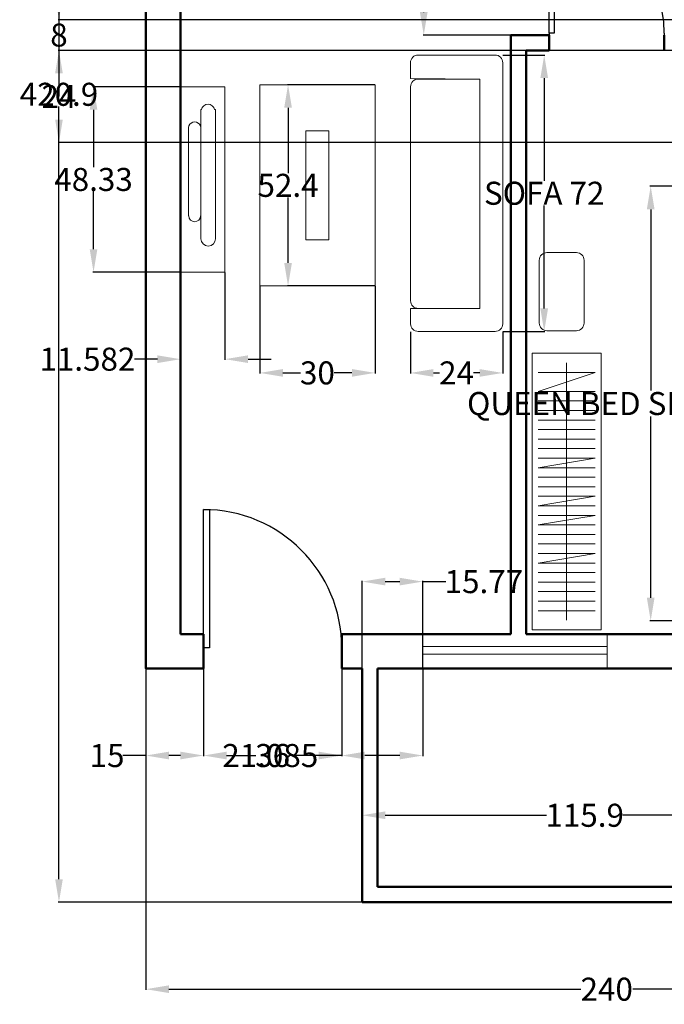
# Model space of a CAD drawing. Units: inches. Extents: x -8 to 300, y -428 to 46.
# Tile 1 of 4: x -8 to 160, y -428 to -172. Entities that reach past the tile are written whole.
import ezdxf

# ---------------------------------------------------------------- set-up
doc = ezdxf.new("R2010")
doc.units = ezdxf.units.IN
doc.header["$MEASUREMENT"] = 0
for name, color, linetype, lineweight in [('A-ANNO-DIMS', 2, 'Continuous', 18), ('A-DOOR', 3, 'Continuous', 25), ('A-EQPM', 8, 'Continuous', 18), ('A-FLOR-CASE', 9, 'Continuous', 18), ('A-FURN', 8, 'Continuous', 18), ('A-GLAZ', 4, 'Continuous', 18), ('A-WALL', 7, 'Continuous', 50)]:
    doc.layers.add(name, color=color, linetype=linetype, lineweight=lineweight)
doc.styles.get("Standard").update_dxf_attribs({"font": 'arial.ttf'})
doc.dimstyles.get("Standard").update_dxf_attribs({"dimtxt": 6, "dimasz": 6, "dimexe": 0.18, "dimexo": 0.0625, "dimgap": 0.09, "dimtad": 0, "dimtih": 1, "dimtoh": 1, "dimdec": 0, "dimzin": 0, "dimdsep": 46, "dimlunit": 4, "dimtxsty": 'Standard', "dimcen": 0.09, "dimadec": 0, "dimazin": 0, "dimtfac": 1, "dimtdec": 0, "dimtofl": 0, "dimtmove": 0, "dimatfit": 3, "dimfxl": 1, "dimtolj": 1, "dimtzin": 0, "dimarcsym": 0})

# ---------------------------------------------------------------- blocks, each defined once
blk = doc.blocks.new('*U2')
for p, q in [((0, 0), (0, -6)), ((40, 0), (40, -6))]:
    blk.add_line(p, q)
blk.add_lwpolyline([(0, 0), (0, 40), (1.75, 40), (1.75, 0)], close=True)
blk.add_arc((0, 0), 40, 0, 90)
blk = doc.blocks.new('SOFA')
for p, q in [((1.98, 72), (22, 72)), ((-0.06, 65.91), (-0.02, 70.02)), ((24, 70), (24, 2)), ((18, 65.74), (-0.06, 65.91)), ((18, 6), (18, 65.74)), ((0, 2), (0, 6)), ((0, 6), (18, 6)), ((22, 0), (2, 0))]:
    blk.add_line(p, q)
blk.add_lwpolyline([(18, 65.74), (2, 65.74, 0.414214), (0, 63.74), (0, 8, 0.414214), (2, 6), (18, 6)], format="xyb", close=True)
for centre, start, end in [((1.98, 70), 90, 179.4484), ((22, 70), 0, 90), ((2, 2), 180, 270), ((22, 2), 270, 0)]:
    blk.add_arc(centre, 2, start, end)
blk = doc.blocks.new('*D17')
at = {"layer": 'A-ANNO-DIMS', "color": 0, "lineweight": -2, "transparency": 16777216}
for p, q in [((173.24, -215.1), (156.15, -215.1)), ((156.33, -221.1), (156.33, -268.3)), ((156.33, -322.26), (156.33, -275.06)), ((173.24, -328.26), (156.15, -328.26))]:
    blk.add_line(p, q, dxfattribs=at)
at = {"layer": 'A-ANNO-DIMS', "color": 0, "transparency": 16777216}
for points in [[(155.33, -221.1), (157.33, -221.1), (156.33, -215.1)], [(155.33, -322.26), (157.33, -322.26), (156.33, -328.26)]]:
    blk.add_solid(points, dxfattribs=at)
at = {"layer": 'Defpoints', "color": 0, "transparency": 16777216}
for p in [(173.3, -215.1), (156.33, -328.26), (173.3, -328.26)]:
    blk.add_point(p, dxfattribs=at)
at = {"layer": 'A-ANNO-DIMS', "color": 0, "transparency": 16777216, "insert": (156.33, -271.68), "char_height": 6, "attachment_point": 5}
blk.add_mtext('\\A1;QUEEN BED SET 113 TYP.', dxfattribs=at)
blk = doc.blocks.new('*D29')
at = {"layer": 'A-ANNO-DIMS', "color": 0, "lineweight": -2, "transparency": 16777216}
for p, q in [((117.86, -180.91), (128.78, -180.91)), ((128.6, -186.91), (128.6, -213.72)), ((128.6, -246.91), (128.6, -220.1)), ((117.86, -252.91), (128.78, -252.91))]:
    blk.add_line(p, q, dxfattribs=at)
at = {"layer": 'A-ANNO-DIMS', "color": 0, "transparency": 16777216}
for points in [[(127.6, -186.91), (129.6, -186.91), (128.6, -180.91)], [(127.6, -246.91), (129.6, -246.91), (128.6, -252.91)]]:
    blk.add_solid(points, dxfattribs=at)
at = {"layer": 'Defpoints', "color": 0, "transparency": 16777216}
for p in [(117.8, -180.91), (128.6, -180.91), (117.8, -252.91)]:
    blk.add_point(p, dxfattribs=at)
at = {"layer": 'A-ANNO-DIMS', "color": 0, "transparency": 16777216, "insert": (128.6, -216.91), "char_height": 6, "attachment_point": 5}
blk.add_mtext('\\A1;SOFA 72', dxfattribs=at)
blk = doc.blocks.new('*D30')
at = {"layer": 'A-ANNO-DIMS', "color": 0, "lineweight": -2, "transparency": 16777216}
for p, q in [((93.74, -252.97), (93.74, -263.89)), ((117.8, -252.97), (117.8, -263.89)), ((99.74, -263.71), (101.34, -263.71)), ((111.8, -263.71), (110.19, -263.71))]:
    blk.add_line(p, q, dxfattribs=at)
at = {"layer": 'A-ANNO-DIMS', "color": 0, "transparency": 16777216}
for points in [[(99.74, -262.71), (99.74, -264.71), (93.74, -263.71)], [(111.8, -262.71), (111.8, -264.71), (117.8, -263.71)]]:
    blk.add_solid(points, dxfattribs=at)
at = {"layer": 'Defpoints', "color": 0, "transparency": 16777216}
for p in [(93.74, -252.91), (117.8, -252.91), (117.8, -263.71)]:
    blk.add_point(p, dxfattribs=at)
at = {"layer": 'A-ANNO-DIMS', "color": 0, "transparency": 16777216, "insert": (105.77, -263.71), "char_height": 6, "attachment_point": 5}
blk.add_mtext('\\A1;24', dxfattribs=at)
blk = doc.blocks.new('*D31')
at = {"layer": 'A-ANNO-DIMS', "color": 0, "lineweight": -2, "transparency": 16777216}
for p, q in [((24.88, -340.77), (24.88, -424.4)), ((264.88, -340.77), (264.88, -424.4)), ((30.88, -424.22), (138.12, -424.22)), ((258.88, -424.22), (151.64, -424.22))]:
    blk.add_line(p, q, dxfattribs=at)
at = {"layer": 'A-ANNO-DIMS', "color": 0, "transparency": 16777216}
for points in [[(30.88, -423.22), (30.88, -425.22), (24.88, -424.22)], [(258.88, -423.22), (258.88, -425.22), (264.88, -424.22)]]:
    blk.add_solid(points, dxfattribs=at)
at = {"layer": 'Defpoints', "color": 0, "transparency": 16777216}
for p in [(24.88, -340.71), (264.88, -340.71), (264.88, -424.22)]:
    blk.add_point(p, dxfattribs=at)
at = {"layer": 'A-ANNO-DIMS', "color": 0, "transparency": 16777216, "insert": (144.88, -424.22), "char_height": 6, "attachment_point": 5}
blk.add_mtext('\\A1;240', dxfattribs=at)
blk = doc.blocks.new('*D32')
at = {"layer": 'A-ANNO-DIMS', "color": 0, "lineweight": -2, "transparency": 16777216}
for p, q in [((24.81, 19.29), (2.05, 19.29)), ((2.23, 13.29), (2.23, -187.98)), ((2.23, -395.57), (2.23, -194.29)), ((81.13, -401.57), (2.05, -401.57))]:
    blk.add_line(p, q, dxfattribs=at)
at = {"layer": 'A-ANNO-DIMS', "color": 0, "transparency": 16777216}
for points in [[(1.23, 13.29), (3.23, 13.29), (2.23, 19.29)], [(1.23, -395.57), (3.23, -395.57), (2.23, -401.57)]]:
    blk.add_solid(points, dxfattribs=at)
at = {"layer": 'Defpoints', "color": 0, "transparency": 16777216}
for p in [(24.88, 19.29), (2.23, -401.57), (81.19, -401.57)]:
    blk.add_point(p, dxfattribs=at)
at = {"layer": 'A-ANNO-DIMS', "color": 0, "transparency": 16777216, "insert": (2.23, -191.14), "char_height": 6, "attachment_point": 5}
blk.add_mtext('\\A1;420.9', dxfattribs=at)
blk = doc.blocks.new('*D34')
at = {"layer": 'A-ANNO-DIMS', "color": 0, "lineweight": -2, "transparency": 16777216}
for p, q in [((81.19, -401.51), (81.19, -378.74)), ((87.19, -378.92), (129.21, -378.92)), ((191.09, -378.92), (149.08, -378.92)), ((197.09, -401.51), (197.09, -378.74))]:
    blk.add_line(p, q, dxfattribs=at)
at = {"layer": 'A-ANNO-DIMS', "color": 0, "transparency": 16777216}
for points in [[(87.19, -377.92), (87.19, -379.92), (81.19, -378.92)], [(191.09, -377.92), (191.09, -379.92), (197.09, -378.92)]]:
    blk.add_solid(points, dxfattribs=at)
at = {"layer": 'Defpoints', "color": 0, "transparency": 16777216}
for p in [(197.09, -378.92), (81.19, -401.57), (197.09, -401.57)]:
    blk.add_point(p, dxfattribs=at)
at = {"layer": 'A-ANNO-DIMS', "color": 0, "transparency": 16777216, "insert": (139.14, -378.92), "char_height": 6, "attachment_point": 5}
blk.add_mtext('\\A1;115.9', dxfattribs=at)
blk = doc.blocks.new('*D35')
at = {"layer": 'A-ANNO-DIMS', "color": 0, "lineweight": -2, "transparency": 16777216}
for p, q in [((81.19, -340.64), (81.19, -317.88)), ((96.96, -340.64), (96.96, -317.88)), ((87.19, -318.06), (90.96, -318.06)), ((96.96, -318.06), (102.96, -318.06))]:
    blk.add_line(p, q, dxfattribs=at)
at = {"layer": 'A-ANNO-DIMS', "color": 0, "transparency": 16777216}
for points in [[(87.19, -317.06), (87.19, -319.06), (81.19, -318.06)], [(90.96, -317.06), (90.96, -319.06), (96.96, -318.06)]]:
    blk.add_solid(points, dxfattribs=at)
at = {"layer": 'Defpoints', "color": 0, "transparency": 16777216}
for p in [(96.96, -318.06), (81.19, -340.71), (96.96, -340.71)]:
    blk.add_point(p, dxfattribs=at)
at = {"layer": 'A-ANNO-DIMS', "color": 0, "transparency": 16777216, "insert": (112.89, -318.06), "char_height": 6, "attachment_point": 5}
blk.add_mtext('\\A1;15.77', dxfattribs=at)
blk = doc.blocks.new('*D41')
at = {"layer": 'A-ANNO-DIMS', "color": 0, "lineweight": -2, "transparency": 16777216}
for p, q in [((119.81, -111.71), (97.05, -111.71)), ((97.23, -117.71), (97.23, -140.55)), ((97.23, -169.71), (97.23, -146.86)), ((119.81, -175.71), (97.05, -175.71))]:
    blk.add_line(p, q, dxfattribs=at)
at = {"layer": 'A-ANNO-DIMS', "color": 0, "transparency": 16777216}
for points in [[(96.23, -117.71), (98.23, -117.71), (97.23, -111.71)], [(96.23, -169.71), (98.23, -169.71), (97.23, -175.71)]]:
    blk.add_solid(points, dxfattribs=at)
at = {"layer": 'Defpoints', "color": 0, "transparency": 16777216}
for p in [(97.23, -111.71), (119.88, -111.71), (119.88, -175.71)]:
    blk.add_point(p, dxfattribs=at)
at = {"layer": 'A-ANNO-DIMS', "color": 0, "transparency": 16777216, "insert": (97.23, -143.71), "char_height": 6, "attachment_point": 5}
blk.add_mtext('\\A1;64', dxfattribs=at)
blk = doc.blocks.new('*D42')
at = {"layer": 'A-ANNO-DIMS', "color": 0, "lineweight": -2, "transparency": 16777216}
for p, q in [((39.88, -340.77), (39.88, -363.54)), ((75.88, -340.77), (75.88, -363.54)), ((45.88, -363.36), (53.49, -363.36)), ((69.88, -363.36), (62.26, -363.36))]:
    blk.add_line(p, q, dxfattribs=at)
at = {"layer": 'A-ANNO-DIMS', "color": 0, "transparency": 16777216}
for points in [[(45.88, -362.36), (45.88, -364.36), (39.88, -363.36)], [(69.88, -362.36), (69.88, -364.36), (75.88, -363.36)]]:
    blk.add_solid(points, dxfattribs=at)
at = {"layer": 'Defpoints', "color": 0, "transparency": 16777216}
for p in [(39.88, -340.71), (75.88, -340.71), (39.88, -363.36)]:
    blk.add_point(p, dxfattribs=at)
at = {"layer": 'A-ANNO-DIMS', "color": 0, "transparency": 16777216, "insert": (57.88, -363.36), "char_height": 6, "attachment_point": 5}
blk.add_mtext('\\A1;36', dxfattribs=at)
blk = doc.blocks.new('*D43')
at = {"layer": 'A-ANNO-DIMS', "color": 0, "lineweight": -2, "transparency": 16777216}
for p, q in [((24.88, -340.77), (24.88, -363.54)), ((39.88, -340.77), (39.88, -363.54)), ((24.88, -363.36), (18.88, -363.36)), ((33.88, -363.36), (30.88, -363.36))]:
    blk.add_line(p, q, dxfattribs=at)
at = {"layer": 'A-ANNO-DIMS', "color": 0, "transparency": 16777216}
for points in [[(30.88, -362.36), (30.88, -364.36), (24.88, -363.36)], [(33.88, -362.36), (33.88, -364.36), (39.88, -363.36)]]:
    blk.add_solid(points, dxfattribs=at)
at = {"layer": 'Defpoints', "color": 0, "transparency": 16777216}
for p in [(24.88, -340.71), (39.88, -340.71), (24.88, -363.36)]:
    blk.add_point(p, dxfattribs=at)
at = {"layer": 'A-ANNO-DIMS', "color": 0, "transparency": 16777216, "insert": (14.75, -363.36), "char_height": 6, "attachment_point": 5}
blk.add_mtext('\\A1;15', dxfattribs=at)
blk = doc.blocks.new('*D51')
at = {"layer": 'A-ANNO-DIMS', "color": 0, "lineweight": -2, "transparency": 16777216}
for p, q in [((75.88, -340.77), (75.88, -363.54)), ((96.96, -340.77), (96.96, -363.54)), ((75.88, -363.36), (69.88, -363.36)), ((90.96, -363.36), (81.88, -363.36))]:
    blk.add_line(p, q, dxfattribs=at)
at = {"layer": 'A-ANNO-DIMS', "color": 0, "transparency": 16777216}
for points in [[(81.88, -362.36), (81.88, -364.36), (75.88, -363.36)], [(90.96, -362.36), (90.96, -364.36), (96.96, -363.36)]]:
    blk.add_solid(points, dxfattribs=at)
at = {"layer": 'Defpoints', "color": 0, "transparency": 16777216}
for p in [(75.88, -340.71), (96.96, -340.71), (75.88, -363.36)]:
    blk.add_point(p, dxfattribs=at)
at = {"layer": 'A-ANNO-DIMS', "color": 0, "transparency": 16777216, "insert": (57.26, -363.36), "char_height": 6, "attachment_point": 5}
blk.add_mtext('\\A1;21.085', dxfattribs=at)
blk = doc.blocks.new('*D58')
at = {"layer": 'A-ANNO-DIMS', "color": 0, "lineweight": -2, "transparency": 16777216}
for p, q in [((2.225934, -165.706734), (2.225934, -159.706734)), ((181.813434, -171.706734), (2.045934, -171.706734)), ((177.813434, -179.706734), (2.045934, -179.706734)), ((2.225934, -185.706734), (2.225934, -191.706734))]:
    blk.add_line(p, q, dxfattribs=at)
at = {"layer": 'A-ANNO-DIMS', "color": 0, "transparency": 16777216}
for points in [[(1.225934, -165.706734), (3.225934, -165.706734), (2.225934, -171.706734)], [(1.225934, -185.706734), (3.225934, -185.706734), (2.225934, -179.706734)]]:
    blk.add_solid(points, dxfattribs=at)
at = {"layer": 'Defpoints', "color": 0, "transparency": 16777216}
for p in [(2.225934, -171.706734), (181.875934, -171.706734), (177.875934, -179.706734)]:
    blk.add_point(p, dxfattribs=at)
at = {"layer": 'A-ANNO-DIMS', "color": 0, "transparency": 16777216, "insert": (2.225934, -175.706734), "char_height": 6, "attachment_point": 5}
blk.add_mtext('\\A1;8', dxfattribs=at)
blk = doc.blocks.new('*D59')
at = {"layer": 'A-ANNO-DIMS', "color": 0, "lineweight": -2, "transparency": 16777216}
for p, q in [((177.81, -179.71), (2.05, -179.71)), ((2.23, -185.71), (2.23, -188.6)), ((2.23, -197.71), (2.23, -194.81)), ((177.81, -203.71), (2.05, -203.71))]:
    blk.add_line(p, q, dxfattribs=at)
at = {"layer": 'A-ANNO-DIMS', "color": 0, "transparency": 16777216}
for points in [[(1.23, -185.71), (3.23, -185.71), (2.23, -179.71)], [(1.23, -197.71), (3.23, -197.71), (2.23, -203.71)]]:
    blk.add_solid(points, dxfattribs=at)
at = {"layer": 'Defpoints', "color": 0, "transparency": 16777216}
for p in [(2.23, -179.71), (177.88, -179.71), (177.88, -203.71)]:
    blk.add_point(p, dxfattribs=at)
at = {"layer": 'A-ANNO-DIMS', "color": 0, "transparency": 16777216, "insert": (2.23, -191.71), "char_height": 6, "attachment_point": 5}
blk.add_mtext('\\A1;24', dxfattribs=at)
blk = doc.blocks.new('*D65')
at = {"layer": 'A-ANNO-DIMS', "color": 0, "lineweight": -2, "transparency": 16777216}
for p, q in [((54.54, -241.11), (54.54, -263.88)), ((84.54, -241.11), (84.54, -263.88)), ((60.54, -263.7), (65.17, -263.7)), ((78.54, -263.7), (73.92, -263.7))]:
    blk.add_line(p, q, dxfattribs=at)
at = {"layer": 'A-ANNO-DIMS', "color": 0, "transparency": 16777216}
for points in [[(60.54, -262.7), (60.54, -264.7), (54.54, -263.7)], [(78.54, -262.7), (78.54, -264.7), (84.54, -263.7)]]:
    blk.add_solid(points, dxfattribs=at)
at = {"layer": 'Defpoints', "color": 0, "transparency": 16777216}
for p in [(54.54, -241.05), (84.54, -241.05), (54.54, -263.7)]:
    blk.add_point(p, dxfattribs=at)
at = {"layer": 'A-ANNO-DIMS', "color": 0, "transparency": 16777216, "insert": (69.54, -263.7), "char_height": 6, "attachment_point": 5}
blk.add_mtext('\\A1;30', dxfattribs=at)
blk = doc.blocks.new('*D66')
at = {"layer": 'A-ANNO-DIMS', "color": 0, "lineweight": -2, "transparency": 16777216}
for p, q in [((84.48, -188.65), (61.71, -188.65)), ((61.89, -194.65), (61.89, -211.7)), ((61.89, -235.05), (61.89, -218)), ((84.48, -241.05), (61.71, -241.05))]:
    blk.add_line(p, q, dxfattribs=at)
at = {"layer": 'A-ANNO-DIMS', "color": 0, "transparency": 16777216}
for points in [[(60.89, -194.65), (62.89, -194.65), (61.89, -188.65)], [(60.89, -235.05), (62.89, -235.05), (61.89, -241.05)]]:
    blk.add_solid(points, dxfattribs=at)
at = {"layer": 'Defpoints', "color": 0, "transparency": 16777216}
for p in [(61.89, -188.65), (84.54, -188.65), (84.54, -241.05)]:
    blk.add_point(p, dxfattribs=at)
at = {"layer": 'A-ANNO-DIMS', "color": 0, "transparency": 16777216, "insert": (61.89, -214.85), "char_height": 6, "attachment_point": 5}
blk.add_mtext('\\A1;52.4', dxfattribs=at)
blk = doc.blocks.new('*D69')
at = {"layer": 'A-ANNO-DIMS', "color": 0, "lineweight": -2, "transparency": 16777216}
for p, q in [((33.88, -237.55), (33.88, -260.31)), ((45.46, -237.55), (45.46, -260.31)), ((27.88, -260.13), (21.88, -260.13)), ((51.46, -260.13), (57.46, -260.13))]:
    blk.add_line(p, q, dxfattribs=at)
at = {"layer": 'A-ANNO-DIMS', "color": 0, "transparency": 16777216}
for points in [[(27.88, -259.13), (27.88, -261.13), (33.88, -260.13)], [(51.46, -259.13), (51.46, -261.13), (45.46, -260.13)]]:
    blk.add_solid(points, dxfattribs=at)
at = {"layer": 'Defpoints', "color": 0, "transparency": 16777216}
for p in [(33.88, -237.48), (45.46, -237.48), (33.88, -260.13)]:
    blk.add_point(p, dxfattribs=at)
at = {"layer": 'A-ANNO-DIMS', "color": 0, "transparency": 16777216, "insert": (9.64, -260.13), "char_height": 6, "attachment_point": 5}
blk.add_mtext('\\A1;11.582', dxfattribs=at)
blk = doc.blocks.new('*D70')
at = {"layer": 'A-ANNO-DIMS', "color": 0, "lineweight": -2, "transparency": 16777216}
for p, q in [((33.81, -189.16), (11.05, -189.16)), ((11.23, -195.16), (11.23, -210.16)), ((11.23, -231.48), (11.23, -216.47)), ((33.81, -237.48), (11.05, -237.48))]:
    blk.add_line(p, q, dxfattribs=at)
at = {"layer": 'A-ANNO-DIMS', "color": 0, "transparency": 16777216}
for points in [[(10.23, -195.16), (12.23, -195.16), (11.23, -189.16)], [(10.23, -231.48), (12.23, -231.48), (11.23, -237.48)]]:
    blk.add_solid(points, dxfattribs=at)
at = {"layer": 'Defpoints', "color": 0, "transparency": 16777216}
for p in [(11.23, -189.16), (33.88, -189.16), (33.88, -237.48)]:
    blk.add_point(p, dxfattribs=at)
at = {"layer": 'A-ANNO-DIMS', "color": 0, "transparency": 16777216, "insert": (11.23, -213.32), "char_height": 6, "attachment_point": 5}
blk.add_mtext('\\A1;48.33', dxfattribs=at)

msp = doc.modelspace()

# ---------------------------------------------------------------- linework, layer by layer
at = {"layer": 'A-EQPM'}
for points in [[(39.1872, -228.7514), (39.1471, -228.7514), (39.1471, -195.1143), (39.3221, -195.1143)], [(42.7679, -195.1143), (43.0294, -195.1143), (43.0294, -228.7514), (42.9894, -228.7514)], [(36.0319, -222.7995), (35.9752, -222.7995), (35.9752, -199.9638)], [(39.1471, -199.9638), (39.1471, -222.7995), (39.0904, -222.7995)]]:
    msp.add_lwpolyline(points, dxfattribs=at)
for centre, radius, start, end in [((41.045, -195.4778), 1.7608, 11.912641, 168.087359), ((37.5611, -199.9638), 1.6144, 349.230662, 190.769338), ((37.5611, -222.7995), 1.5292, 180, 0), ((41.0883, -228.7514), 1.9011, 180, 0)]:
    msp.add_arc(centre, radius, start, end, dxfattribs=at)
at = {"layer": 'A-FLOR-CASE'}
for p, q in [((134.4317, -261.0871), (134.4317, -328.1216)), ((141.8633, -263.5699), (127.0395, -263.5699)), ((141.8633, -263.5699), (127.0395, -268.5354)), ((141.8633, -268.5354), (127.0395, -268.5354)), ((141.8633, -271.0181), (127.0395, -271.0181)), ((141.8633, -273.5009), (127.0395, -273.5009)), ((141.8633, -275.9837), (127.0395, -275.9837)), ((141.8633, -278.4664), (127.0395, -278.4664)), ((141.8633, -280.9492), (127.0395, -280.9492)), ((141.8633, -283.4319), (127.0395, -283.4319)), ((141.8633, -285.9147), (127.0395, -285.9147)), ((141.8633, -285.9147), (127.0395, -288.3975)), ((141.8633, -288.3975), (127.0395, -288.3975)), ((141.8633, -290.8802), (127.0395, -290.8802)), ((141.8633, -293.363), (127.0395, -293.363)), ((141.8633, -295.8457), (127.0395, -295.8457)), ((141.8633, -295.8457), (127.0395, -298.3285)), ((141.8633, -298.3285), (127.0395, -298.3285)), ((141.8633, -300.8112), (127.0395, -300.8112)), ((141.8633, -300.8112), (127.0395, -303.294)), ((141.8633, -303.294), (127.0395, -303.294)), ((141.8633, -305.7768), (127.0395, -305.7768)), ((141.8633, -308.2595), (127.0395, -308.2595)), ((141.8633, -310.7423), (127.0395, -310.7423)), ((141.8633, -310.7423), (127.0395, -313.225)), ((141.8633, -313.225), (127.0395, -313.225)), ((141.8633, -315.7078), (127.0395, -315.7078)), ((141.8633, -318.1906), (127.0395, -318.1906)), ((141.8633, -320.6733), (127.0395, -320.6733)), ((141.8633, -323.1561), (127.0395, -323.1561)), ((141.8633, -325.6388), (127.0395, -325.6388))]:
    msp.add_line(p, q, dxfattribs=at)
msp.add_lwpolyline([(125.4317, -330.6043), (125.4317, -258.6043), (143.4317, -258.6043), (143.4317, -330.6043), (125.4317, -330.6043), (143.4317, -330.6043)], dxfattribs=at)
at = {"layer": 'A-FURN'}
for points in [[(33.8759, -189.1553), (45.4578, -189.1553), (45.4578, -237.4828), (33.8759, -237.4828)], [(54.5441, -188.6472), (84.5441, -188.6472), (84.5441, -241.0503), (54.5441, -241.0503)], [(66.5441, -200.6472), (72.5441, -200.6472), (72.5441, -229.0503), (66.5441, -229.0503)]]:
    msp.add_lwpolyline(points, close=True, dxfattribs=at)
msp.add_lwpolyline([(129.3248, -232.355), (136.9691, -232.355, -0.41421356), (138.9691, -234.355), (138.9691, -250.706, -0.41421356), (136.9691, -252.706), (129.3248, -252.706, -0.41421356), (127.3248, -250.706), (127.3248, -234.355, -0.41421356)], format="xyb", close=True, dxfattribs=at)
at = {"layer": 'A-GLAZ'}
for p, q in [((96.9608, -340.7067), (96.9608, -331.7067)), ((144.9608, -331.4976), (144.9608, -340.4976)), ((96.9608, -334.9976), (144.9608, -334.9976)), ((96.9608, -336.9976), (144.9608, -336.9976))]:
    msp.add_line(p, q, dxfattribs=at)
at = {"layer": 'A-WALL'}
for p, q in [((33.8759, -331.7067), (33.8759, -85.7067)), ((119.8759, -209.7067), (119.8759, -175.7067)), ((123.8759, -175.7067), (119.8759, -175.7067)), ((123.8759, -175.7067), (129.8759, -175.7067)), ((129.8759, -179.7067), (129.8759, -175.7067)), ((159.8759, -179.7067), (159.8759, -175.7067)), ((123.8759, -209.7067), (123.8759, -179.7067)), ((129.8759, -179.7067), (123.8759, -179.7067)), ((119.8759, -209.7067), (119.8759, -331.7067)), ((123.8759, -213.7067), (123.8759, -209.7067)), ((123.8759, -213.7067), (123.8759, -331.7067)), ((39.8759, -331.7067), (33.8759, -331.7067)), ((39.8759, -331.7067), (39.8759, -340.7067)), ((119.8759, -331.7067), (75.8759, -331.7067)), ((75.8759, -331.7067), (75.8759, -340.7067)), ((255.8759, -331.7067), (123.8759, -331.7067)), ((81.1915, -401.5677), (81.1915, -340.7067)), ((85.1915, -397.5677), (85.1915, -340.7067)), ((85.1915, -340.7067), (193.0947, -340.7067)), ((193.0947, -397.5677), (85.1915, -397.5677)), ((197.0947, -401.5677), (81.1915, -401.5677))]:
    msp.add_line(p, q, dxfattribs=at)
for points in [[(39.8759, -340.7067), (24.8759, -340.7067), (24.8759, 19.2933), (264.8759, 19.2933), (264.8759, -340.7067), (197.0947, -340.7067)], [(81.1915, -340.7067), (75.8759, -340.7067)]]:
    msp.add_lwpolyline(points, dxfattribs=at)

# ---------------------------------------------------------------- block references
at = {"layer": 'A-DOOR'}
for p, xscale, yscale, zscale in [((129.8759, -175.2067), 0.75, 0.75, 0.75), ((39.8759, -335.3067), 0.9, 0.9, 0.9)]:
    msp.add_blockref('*U2', p, dxfattribs=dict(at, xscale=xscale, yscale=yscale, zscale=zscale))
at = {"layer": 'A-FURN'}
msp.add_blockref('SOFA', (93.7967, -252.91), dxfattribs=at)

# ---------------------------------------------------------------- dimensions: what is measured, and where the dimension line sits
at = {"layer": 'A-ANNO-DIMS'}
for base, p1, p2, angle, override, picture, middle in [((2.2259, -401.5677), (24.8759, 19.2933), (81.1915, -401.5677), 90, {"dimdec": 1, "dimlfac": 1, "dimrnd": 0, "dimzin": 0, "dimdsep": 46, "dimlunit": 2}, '*D32', (2.2259, -191.1372)), ((97.2259, -111.7067), (119.8759, -175.7067), (119.8759, -111.7067), 90, {"dimdec": 0, "dimlfac": 1, "dimrnd": 0, "dimzin": 0, "dimdsep": 46, "dimlunit": 2}, '*D41', (97.2259, -143.7067)), ((2.2259, -171.7067), (177.8759, -179.7067), (181.8759, -171.7067), 90, {"dimdec": 0, "dimlfac": 1, "dimrnd": 0, "dimzin": 0, "dimdsep": 46, "dimlunit": 2}, '*D58', (2.2259, -175.7067)), ((2.2259, -179.7067), (177.8759, -203.7067), (177.8759, -179.7067), 90, {"dimdec": 0, "dimlfac": 1, "dimrnd": 0, "dimzin": 0, "dimdsep": 46, "dimlunit": 2}, '*D59', (2.2259, -191.7067)), ((11.2259, -189.1553), (33.8759, -237.4828), (33.8759, -189.1553), 90, {"dimdec": 2, "dimlfac": 1, "dimrnd": 0, "dimzin": 0, "dimdsep": 46, "dimlunit": 2}, '*D70', (11.2259, -213.319)), ((61.8941, -188.6472), (84.5441, -241.0503), (84.5441, -188.6472), 90, {"dimdec": 1, "dimlfac": 1, "dimrnd": 0, "dimzin": 0, "dimdsep": 46, "dimlunit": 2}, '*D66', (61.8941, -214.8487)), ((33.8759, -260.1328), (45.4578, -237.4828), (33.8759, -237.4828), 180, {"dimdec": 3, "dimlfac": 1, "dimrnd": 0, "dimzin": 0, "dimdsep": 46, "dimlunit": 2}, '*D69', (9.6447, -260.1328)), ((54.5441, -263.7003), (84.5441, -241.0503), (54.5441, -241.0503), 180, {"dimdec": 0, "dimlfac": 1, "dimrnd": 0, "dimzin": 0, "dimdsep": 46, "dimlunit": 2}, '*D65', (69.5441, -263.7003)), ((24.8759, -363.3567), (39.8759, -340.7067), (24.8759, -340.7067), 180, {"dimdec": 0, "dimlfac": 1, "dimrnd": 0, "dimzin": 0, "dimdsep": 46, "dimlunit": 2}, '*D43', (14.7484, -363.3567)), ((39.8759, -363.3567), (75.8759, -340.7067), (39.8759, -340.7067), 180, {"dimdec": 0, "dimlfac": 1, "dimrnd": 0, "dimzin": 0, "dimdsep": 46, "dimlunit": 2}, '*D42', (57.8759, -363.3567)), ((75.8759, -363.3567), (96.9608, -340.7067), (75.8759, -340.7067), 180, {"dimdec": 3, "dimlfac": 1, "dimrnd": 0, "dimzin": 0, "dimdsep": 46, "dimlunit": 2}, '*D51', (57.258, -363.3567))]:
    dim = msp.add_linear_dim(base=base, p1=p1, p2=p2, angle=angle, dimstyle='Standard', override=override, dxfattribs=at)
    dim.commit()
    dim.dimension.update_dxf_attribs({"geometry": picture, "text_midpoint": middle})
for base, p1, p2, angle, text, picture, middle in [((128.5967, -180.91), (117.7967, -252.91), (117.7967, -180.91), 90, 'SOFA <>', '*D29', (128.5967, -216.91)), ((156.3284, -328.262), (173.3035, -215.0951), (173.3035, -328.262), 270, 'QUEEN BED SET <> TYP.', '*D17', (156.3284, -271.6785))]:
    dim = msp.add_linear_dim(base=base, p1=p1, p2=p2, angle=angle, text=text, dimstyle='Standard', override={"dimdec": 0, "dimlfac": 1, "dimrnd": 0, "dimzin": 0, "dimdsep": 46, "dimlunit": 2}, dxfattribs=at)
    dim.commit()
    dim.dimension.update_dxf_attribs({"geometry": picture, "text_midpoint": middle})
for base, p1, p2, override, picture, middle in [((117.7967, -263.71), (93.7381, -252.91), (117.7967, -252.91), {"dimdec": 0, "dimlfac": 1, "dimrnd": 0, "dimzin": 0, "dimdsep": 46, "dimlunit": 2}, '*D30', (105.7674, -263.71)), ((96.9608, -318.0567), (81.1915, -340.7067), (96.9608, -340.7067), {"dimdec": 2, "dimlfac": 1, "dimrnd": 0, "dimzin": 0, "dimdsep": 46, "dimlunit": 2}, '*D35', (112.8919, -318.0567)), ((264.8759, -424.2177), (24.8759, -340.7067), (264.8759, -340.7067), {"dimdec": 0, "dimlfac": 1, "dimrnd": 0, "dimzin": 0, "dimdsep": 46, "dimlunit": 2}, '*D31', (144.8759, -424.2177)), ((197.0947, -378.9177), (81.1915, -401.5677), (197.0947, -401.5677), {"dimdec": 1, "dimlfac": 1, "dimrnd": 0, "dimzin": 0, "dimdsep": 46, "dimlunit": 2}, '*D34', (139.1431, -378.9177))]:
    dim = msp.add_linear_dim(base=base, p1=p1, p2=p2, dimstyle='Standard', override=override, dxfattribs=at)
    dim.commit()
    dim.dimension.update_dxf_attribs({"geometry": picture, "text_midpoint": middle})

doc.saveas('drawing.dxf')
